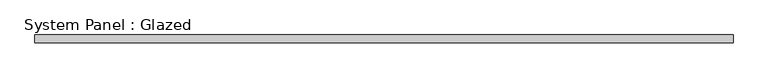
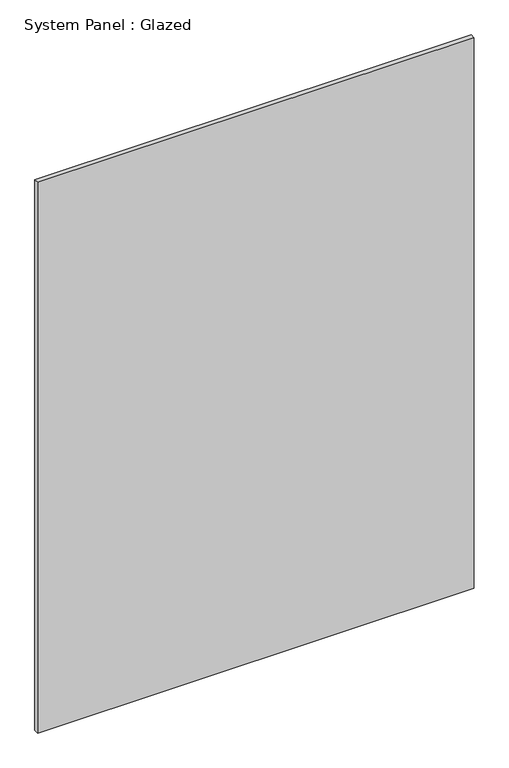
"""IFC4 building model written with IfcOpenShell, lengths in millimetres: plate geometry, System Panel : Glazed."""

from ifc_helpers import new_model, si_unit, origin, origin_with_axes, place, context, project, spatial, polyline, outline, extrude, source, transform, mapped, element, save


def system_panel_glazed_9d4ca976(model_context):
    return source(origin(), model_context, "Body", "SweptSolid", [
        extrude(outline(polyline([(1143.0, 19.05), (-1143.0, 19.05), (-1143.0, 44.45), (1143.0, 44.45), (1143.0, 19.05)])), origin_with_axes(), (0.0, 0.0, 1.0), 3048.0),
    ])


if __name__ == "__main__":
    model = new_model("IFC4")
    model_context = context("Model", 3, world=origin())
    ifc_project = project(units=[si_unit("LENGTHUNIT", "METRE", prefix="MILLI")], contexts=[model_context])
    site = spatial("IfcSite", under=ifc_project)
    building = spatial("IfcBuilding", under=site)
    placement = place(None, origin())
    system_panel_glazed_shape = system_panel_glazed_9d4ca976(model_context)
    element("IfcPlate", 1, ObjectType="System Panel : Glazed", at=placement, inside=building, context=model_context, shape_type="MappedRepresentation", body=[
        mapped(system_panel_glazed_shape, transform((0.0, 0.0, 0.0), x_axis=(1.0, 0.0, 0.0), y_axis=(0.0, 1.0, 0.0), z_axis=(0.0, 0.0, 1.0))),
    ])
    save(model, "model.ifc")

# Revit data of these elements
# Type "System Panel : Glazed"
#   Construction Type Id = "GSP4R"
#   Analytic Construction = "1/8 in Pilkington single glazing"
#   Visual Light Transmittance = 0.9
#   Solar Heat Gain Coefficient = 0.86
#   Heat Transfer Coefficient (U) = 1.18115 BTU/(h·ft²·°F)
#   Define Thermal Properties by = 1
# Element 1 (IfcPlate, "System Panel : Glazed")
#   Materials on its faces: "Glass"
# Materials
#   "Glass": class "Glass", colour RGB 0 128 192, transparency 0.75, Description = "Soda Lime Glass", Cost = 0
